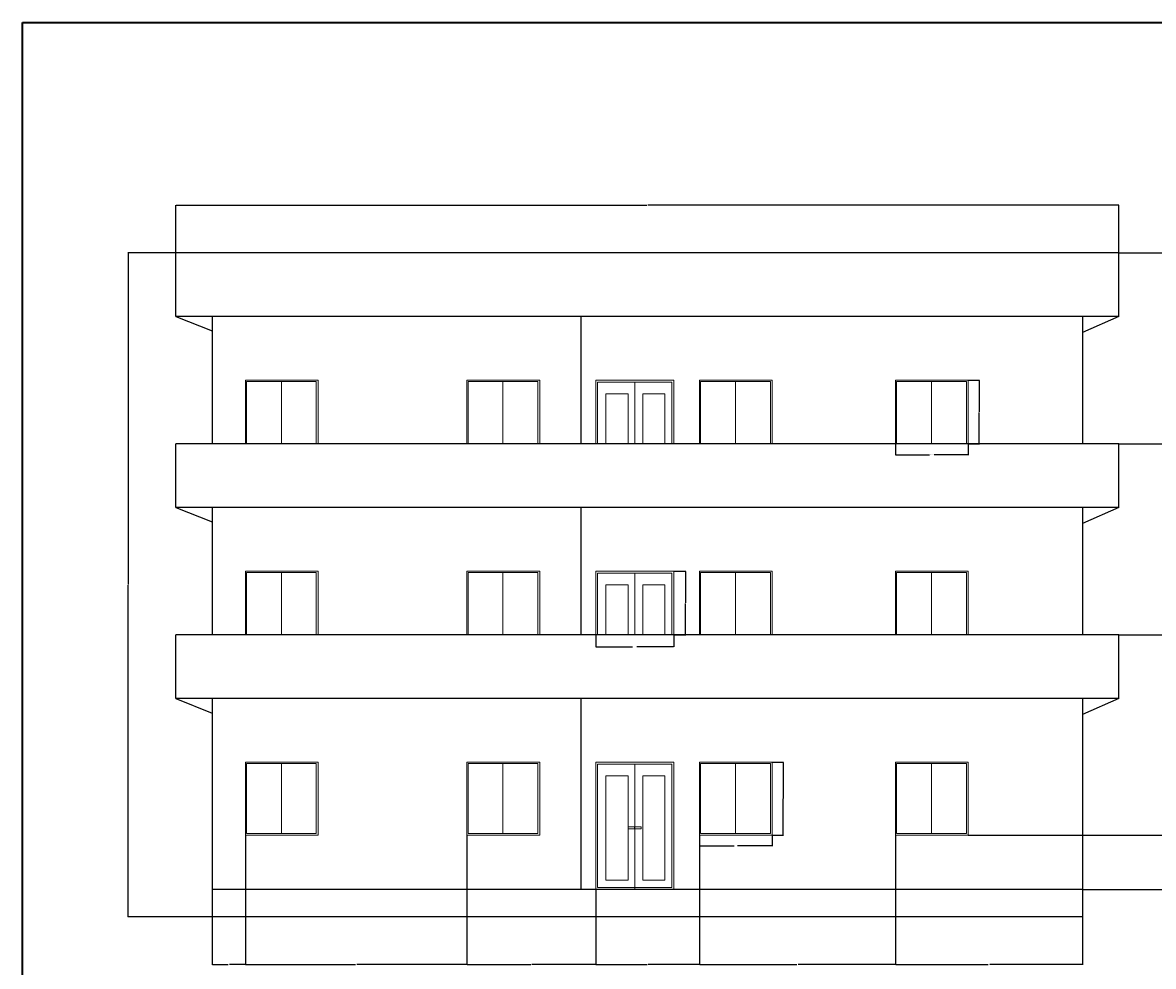
# Model space of a CAD drawing. Units: inches. Extents: x 1824 to 3509, y 619 to 2294.
# Tile 8 of 12: x 1824 to 2570, y 1671 to 2294. Entities that reach past the tile are written whole.
import ezdxf

# ---------------------------------------------------------------- set-up
doc = ezdxf.new("R2010")
doc.units = ezdxf.units.IN
for name, color, linetype, lineweight in [('A-ANNO-DIMS', 2, 'Continuous', 18), ('A-ANNO-TTLB', 7, 'Continuous', 35), ('A-ELEV', 7, 'Continuous', 25), ('A-ELEV-DOOR', 3, 'Continuous', 18), ('A-ELEV-GLAZ', 4, 'Continuous', 18)]:
    doc.layers.add(name, color=color, linetype=linetype, lineweight=lineweight)
doc.styles.get("Standard").update_dxf_attribs({"font": 'arial.ttf'})
doc.dimstyles.get("Standard").update_dxf_attribs({"dimtxt": 0.18, "dimasz": 0.18, "dimexe": 0.18, "dimexo": 0.0625, "dimgap": 0.09, "dimtad": 0, "dimtih": 1, "dimtoh": 1, "dimdec": 4, "dimzin": 0, "dimdsep": 46, "dimtxsty": 'Standard', "dimcen": 0.09, "dimadec": 0, "dimazin": 0, "dimtfac": 1, "dimtdec": 4, "dimtofl": 0, "dimtmove": 0, "dimatfit": 3, "dimfxl": 1, "dimtolj": 1, "dimtzin": 0, "dimarcsym": 0})

# ---------------------------------------------------------------- blocks, each defined once
blk = doc.blocks.new('WIN-ELEV-UPPER')
for p, q in [((0, 42), (0, 0)), ((48, 42), (0, 42)), ((23.74, 41.26), (23.74, 0)), ((48, 42), (48, 0))]:
    blk.add_line(p, q)
blk.add_lwpolyline([(0.72, 0), (0.72, 41.26), (46.77, 41.26), (46.77, 0)])
blk = doc.blocks.new('WIN-ELEV-48')
for p, q in [((0, 48), (0, 0)), ((48, 48), (0, 48)), ((23.74, 47.26), (23.74, 1.1)), ((48, 48), (48, 0)), ((48, 0), (0, 0))]:
    blk.add_line(p, q)
blk.add_lwpolyline([(0.72, 47.26), (46.77, 47.26), (46.77, 1.1), (0.72, 1.1)], close=True)
blk = doc.blocks.new('DOOR-ELEV-UPPER')
for p, q in [((0, 42), (0, 0)), ((51.54, 42), (0, 42)), ((25.72, 40.74), (25.72, 0)), ((51.54, 42), (51.54, 0))]:
    blk.add_line(p, q)
for points in [[(1.26, 0), (1.26, 40.74), (50.17, 40.74), (50.17, 0)], [(6.64, 0), (6.64, 33.08), (21.32, 33.08), (21.32, 0)], [(31.02, 0), (31.02, 33.08), (45.71, 33.08), (45.71, 0)]]:
    blk.add_lwpolyline(points)
blk = doc.blocks.new('*D36')
at = {"layer": 'A-ANNO-DIMS', "color": 0, "lineweight": -2, "transparency": 16777216}
for p, q in [((2399.66, 2015.69), (2399.66, 2008.37)), ((2447.66, 2015.69), (2447.66, 2008.37)), ((2399.84, 2008.55), (2422.08, 2008.55)), ((2447.48, 2008.55), (2425.24, 2008.55))]:
    blk.add_line(p, q, dxfattribs=at)
at = {"layer": 'A-ANNO-DIMS', "color": 0, "transparency": 16777216}
for points in [[(2399.84, 2008.58), (2399.84, 2008.52), (2399.66, 2008.55)], [(2447.48, 2008.58), (2447.48, 2008.52), (2447.66, 2008.55)]]:
    blk.add_solid(points, dxfattribs=at)
at = {"layer": 'Defpoints', "color": 0, "transparency": 16777216}
for p in [(2399.66, 2015.75), (2447.66, 2015.75), (2447.66, 2008.55)]:
    blk.add_point(p, dxfattribs=at)
at = {"layer": 'A-ANNO-DIMS', "color": 0, "transparency": 16777216, "insert": (2423.66, 2008.55), "char_height": 0.18, "attachment_point": 5}
blk.add_mtext('\\A1;UPPER WINDOW 48 TYP.', dxfattribs=at)
blk = doc.blocks.new('*D37')
at = {"layer": 'A-ANNO-DIMS', "color": 0, "lineweight": -2, "transparency": 16777216}
for p, q in [((2447.72, 2057.75), (2455.04, 2057.75)), ((2454.86, 2057.57), (2454.86, 2036.93)), ((2454.86, 2015.93), (2454.86, 2036.57)), ((2447.72, 2015.75), (2455.04, 2015.75))]:
    blk.add_line(p, q, dxfattribs=at)
at = {"layer": 'A-ANNO-DIMS', "color": 0, "transparency": 16777216}
for points in [[(2454.83, 2057.57), (2454.89, 2057.57), (2454.86, 2057.75)], [(2454.83, 2015.93), (2454.89, 2015.93), (2454.86, 2015.75)]]:
    blk.add_solid(points, dxfattribs=at)
at = {"layer": 'Defpoints', "color": 0, "transparency": 16777216}
for p in [(2447.66, 2057.75), (2454.86, 2057.75), (2447.66, 2015.75)]:
    blk.add_point(p, dxfattribs=at)
at = {"layer": 'A-ANNO-DIMS', "color": 0, "transparency": 16777216, "insert": (2454.86, 2036.75), "char_height": 0.18, "attachment_point": 5}
blk.add_mtext('\\A1;42 TYP.', dxfattribs=at)
blk = doc.blocks.new('*D46')
at = {"layer": 'A-ANNO-DIMS', "color": 0, "lineweight": -2, "transparency": 16777216}
for p, q in [((2270.48, 1757.69), (2270.48, 1750.37)), ((2318.48, 1757.69), (2318.48, 1750.37)), ((2270.66, 1750.55), (2293.37, 1750.55)), ((2318.3, 1750.55), (2295.6, 1750.55))]:
    blk.add_line(p, q, dxfattribs=at)
at = {"layer": 'A-ANNO-DIMS', "color": 0, "transparency": 16777216}
for points in [[(2270.66, 1750.58), (2270.66, 1750.52), (2270.48, 1750.55)], [(2318.3, 1750.58), (2318.3, 1750.52), (2318.48, 1750.55)]]:
    blk.add_solid(points, dxfattribs=at)
at = {"layer": 'Defpoints', "color": 0, "transparency": 16777216}
for p in [(2270.48, 1757.75), (2318.48, 1757.75), (2318.48, 1750.55)]:
    blk.add_point(p, dxfattribs=at)
at = {"layer": 'A-ANNO-DIMS', "color": 0, "transparency": 16777216, "insert": (2294.48, 1750.55), "char_height": 0.18, "attachment_point": 5}
blk.add_mtext('\\A1;WINDOW 48 TYP.', dxfattribs=at)
blk = doc.blocks.new('*D47')
at = {"layer": 'A-ANNO-DIMS', "color": 0, "lineweight": -2, "transparency": 16777216}
for p, q in [((2318.55, 1805.75), (2325.86, 1805.75)), ((2325.68, 1805.57), (2325.68, 1781.93)), ((2325.68, 1757.93), (2325.68, 1781.57)), ((2318.55, 1757.75), (2325.86, 1757.75))]:
    blk.add_line(p, q, dxfattribs=at)
at = {"layer": 'A-ANNO-DIMS', "color": 0, "transparency": 16777216}
for points in [[(2325.65, 1805.57), (2325.71, 1805.57), (2325.68, 1805.75)], [(2325.65, 1757.93), (2325.71, 1757.93), (2325.68, 1757.75)]]:
    blk.add_solid(points, dxfattribs=at)
at = {"layer": 'Defpoints', "color": 0, "transparency": 16777216}
for p in [(2318.48, 1805.75), (2325.68, 1805.75), (2318.48, 1757.75)]:
    blk.add_point(p, dxfattribs=at)
at = {"layer": 'A-ANNO-DIMS', "color": 0, "transparency": 16777216, "insert": (2325.68, 1781.75), "char_height": 0.18, "attachment_point": 5}
blk.add_mtext('\\A1;48 TYP.', dxfattribs=at)
blk = doc.blocks.new('*D86')
at = {"layer": 'A-ANNO-DIMS', "color": 0, "lineweight": -2, "transparency": 16777216}
for p, q in [((2201.98, 1889.69), (2201.98, 1881.84)), ((2253.53, 1889.69), (2253.53, 1881.84)), ((2202.16, 1882.02), (2226.35, 1882.02)), ((2253.35, 1882.02), (2229.16, 1882.02))]:
    blk.add_line(p, q, dxfattribs=at)
at = {"layer": 'A-ANNO-DIMS', "color": 0, "transparency": 16777216}
for points in [[(2202.16, 1882.05), (2202.16, 1881.99), (2201.98, 1882.02)], [(2253.35, 1882.05), (2253.35, 1881.99), (2253.53, 1882.02)]]:
    blk.add_solid(points, dxfattribs=at)
at = {"layer": 'Defpoints', "color": 0, "transparency": 16777216}
for p in [(2201.98, 1889.75), (2253.53, 1889.75), (2253.53, 1882.02)]:
    blk.add_point(p, dxfattribs=at)
at = {"layer": 'A-ANNO-DIMS', "color": 0, "transparency": 16777216, "insert": (2227.76, 1882.02), "char_height": 0.18, "attachment_point": 5}
blk.add_mtext('\\A1;UPPER DOOR 52 TYP.', dxfattribs=at)
blk = doc.blocks.new('*D87')
at = {"layer": 'A-ANNO-DIMS', "color": 0, "lineweight": -2, "transparency": 16777216}
for p, q in [((2253.59, 1931.75), (2261.44, 1931.75)), ((2261.26, 1931.57), (2261.26, 1910.93)), ((2261.26, 1889.93), (2261.26, 1910.57)), ((2253.59, 1889.75), (2261.44, 1889.75))]:
    blk.add_line(p, q, dxfattribs=at)
at = {"layer": 'A-ANNO-DIMS', "color": 0, "transparency": 16777216}
for points in [[(2261.23, 1931.57), (2261.29, 1931.57), (2261.26, 1931.75)], [(2261.23, 1889.93), (2261.29, 1889.93), (2261.26, 1889.75)]]:
    blk.add_solid(points, dxfattribs=at)
at = {"layer": 'Defpoints', "color": 0, "transparency": 16777216}
for p in [(2253.53, 1931.75), (2261.26, 1931.75), (2253.53, 1889.75)]:
    blk.add_point(p, dxfattribs=at)
at = {"layer": 'A-ANNO-DIMS', "color": 0, "transparency": 16777216, "insert": (2261.26, 1910.75), "char_height": 0.18, "attachment_point": 5}
blk.add_mtext('\\A1;42 TYP.', dxfattribs=at)
blk = doc.blocks.new('*D118')
at = {"layer": 'A-ANNO-DIMS', "color": 0, "lineweight": -2, "transparency": 16777216}
for p, q in [((1925.09, 2141.81), (1925.09, 2173.33)), ((1925.27, 2173.15), (2235.8, 2173.15)), ((2546.91, 2173.15), (2236.38, 2173.15)), ((2547.09, 2141.81), (2547.09, 2173.33))]:
    blk.add_line(p, q, dxfattribs=at)
at = {"layer": 'A-ANNO-DIMS', "color": 0, "transparency": 16777216}
for points in [[(1925.27, 2173.18), (1925.27, 2173.12), (1925.09, 2173.15)], [(2546.91, 2173.18), (2546.91, 2173.12), (2547.09, 2173.15)]]:
    blk.add_solid(points, dxfattribs=at)
at = {"layer": 'Defpoints', "color": 0, "transparency": 16777216}
for p in [(2547.09, 2173.15), (1925.09, 2141.75), (2547.09, 2141.75)]:
    blk.add_point(p, dxfattribs=at)
at = {"layer": 'A-ANNO-DIMS', "color": 0, "transparency": 16777216, "insert": (2236.09, 2173.15), "char_height": 0.18, "attachment_point": 5}
blk.add_mtext('\\A1;622', dxfattribs=at)
blk = doc.blocks.new('*D119')
at = {"layer": 'A-ANNO-DIMS', "color": 0, "lineweight": -2, "transparency": 16777216}
for p, q in [((1925.03, 2141.75), (1893.51, 2141.75)), ((1893.69, 2141.57), (1893.69, 1922.93)), ((1893.69, 1703.93), (1893.69, 1922.57)), ((1949.03, 1703.75), (1893.51, 1703.75))]:
    blk.add_line(p, q, dxfattribs=at)
at = {"layer": 'A-ANNO-DIMS', "color": 0, "transparency": 16777216}
for points in [[(1893.66, 2141.57), (1893.72, 2141.57), (1893.69, 2141.75)], [(1893.66, 1703.93), (1893.72, 1703.93), (1893.69, 1703.75)]]:
    blk.add_solid(points, dxfattribs=at)
at = {"layer": 'Defpoints', "color": 0, "transparency": 16777216}
for p in [(1893.69, 2141.75), (1925.09, 2141.75), (1949.09, 1703.75)]:
    blk.add_point(p, dxfattribs=at)
at = {"layer": 'A-ANNO-DIMS', "color": 0, "transparency": 16777216, "insert": (1893.69, 1922.75), "char_height": 0.18, "attachment_point": 5}
blk.add_mtext('\\A1;438', dxfattribs=at)
blk = doc.blocks.new('*D120')
at = {"layer": 'A-ANNO-DIMS', "color": 0, "lineweight": -2, "transparency": 16777216}
for p, q in [((1970.95, 1757.69), (1970.95, 1672.17)), ((1949.09, 1703.69), (1949.09, 1672.17)), ((1949.27, 1672.35), (1959.56, 1672.35)), ((1970.77, 1672.35), (1960.49, 1672.35))]:
    blk.add_line(p, q, dxfattribs=at)
at = {"layer": 'A-ANNO-DIMS', "color": 0, "transparency": 16777216}
for points in [[(1949.27, 1672.38), (1949.27, 1672.32), (1949.09, 1672.35)], [(1970.77, 1672.38), (1970.77, 1672.32), (1970.95, 1672.35)]]:
    blk.add_solid(points, dxfattribs=at)
at = {"layer": 'Defpoints', "color": 0, "transparency": 16777216}
for p in [(1970.95, 1757.75), (1949.09, 1703.75), (1970.95, 1672.35)]:
    blk.add_point(p, dxfattribs=at)
at = {"layer": 'A-ANNO-DIMS', "color": 0, "transparency": 16777216, "insert": (1960.02, 1672.35), "char_height": 0.18, "attachment_point": 5}
blk.add_mtext('\\A1;21.863', dxfattribs=at)
blk = doc.blocks.new('*D121')
at = {"layer": 'A-ANNO-DIMS', "color": 0, "lineweight": -2, "transparency": 16777216}
for p, q in [((1970.95, 1757.69), (1970.95, 1672.17)), ((2117.11, 1757.69), (2117.11, 1672.17)), ((1971.13, 1672.35), (2043.58, 1672.35)), ((2116.93, 1672.35), (2044.49, 1672.35))]:
    blk.add_line(p, q, dxfattribs=at)
at = {"layer": 'A-ANNO-DIMS', "color": 0, "transparency": 16777216}
for points in [[(1971.13, 1672.38), (1971.13, 1672.32), (1970.95, 1672.35)], [(2116.93, 1672.38), (2116.93, 1672.32), (2117.11, 1672.35)]]:
    blk.add_solid(points, dxfattribs=at)
at = {"layer": 'Defpoints', "color": 0, "transparency": 16777216}
for p in [(1970.95, 1757.75), (2117.11, 1757.75), (2117.11, 1672.35)]:
    blk.add_point(p, dxfattribs=at)
at = {"layer": 'A-ANNO-DIMS', "color": 0, "transparency": 16777216, "insert": (2044.03, 1672.35), "char_height": 0.18, "attachment_point": 5}
blk.add_mtext('\\A1;146.16', dxfattribs=at)
blk = doc.blocks.new('*D122')
at = {"layer": 'A-ANNO-DIMS', "color": 0, "lineweight": -2, "transparency": 16777216}
for p, q in [((2117.11, 1757.69), (2117.11, 1672.17)), ((2201.98, 1721.69), (2201.98, 1672.17)), ((2117.29, 1672.35), (2159.15, 1672.35)), ((2201.8, 1672.35), (2159.94, 1672.35))]:
    blk.add_line(p, q, dxfattribs=at)
at = {"layer": 'A-ANNO-DIMS', "color": 0, "transparency": 16777216}
for points in [[(2117.29, 1672.38), (2117.29, 1672.32), (2117.11, 1672.35)], [(2201.8, 1672.38), (2201.8, 1672.32), (2201.98, 1672.35)]]:
    blk.add_solid(points, dxfattribs=at)
at = {"layer": 'Defpoints', "color": 0, "transparency": 16777216}
for p in [(2117.11, 1757.75), (2201.98, 1721.75), (2201.98, 1672.35)]:
    blk.add_point(p, dxfattribs=at)
at = {"layer": 'A-ANNO-DIMS', "color": 0, "transparency": 16777216, "insert": (2159.55, 1672.35), "char_height": 0.18, "attachment_point": 5}
blk.add_mtext('\\A1;84.87', dxfattribs=at)
blk = doc.blocks.new('*D123')
at = {"layer": 'A-ANNO-DIMS', "color": 0, "lineweight": -2, "transparency": 16777216}
for p, q in [((2270.48, 1757.69), (2270.48, 1672.17)), ((2201.98, 1721.69), (2201.98, 1672.17)), ((2202.16, 1672.35), (2235.91, 1672.35)), ((2270.3, 1672.35), (2236.56, 1672.35))]:
    blk.add_line(p, q, dxfattribs=at)
at = {"layer": 'A-ANNO-DIMS', "color": 0, "transparency": 16777216}
for points in [[(2202.16, 1672.38), (2202.16, 1672.32), (2201.98, 1672.35)], [(2270.3, 1672.38), (2270.3, 1672.32), (2270.48, 1672.35)]]:
    blk.add_solid(points, dxfattribs=at)
at = {"layer": 'Defpoints', "color": 0, "transparency": 16777216}
for p in [(2270.48, 1757.75), (2201.98, 1721.75), (2270.48, 1672.35)]:
    blk.add_point(p, dxfattribs=at)
at = {"layer": 'A-ANNO-DIMS', "color": 0, "transparency": 16777216, "insert": (2236.23, 1672.35), "char_height": 0.18, "attachment_point": 5}
blk.add_mtext('\\A1;68.5', dxfattribs=at)
blk = doc.blocks.new('*D124')
at = {"layer": 'A-ANNO-DIMS', "color": 0, "lineweight": -2, "transparency": 16777216}
for p, q in [((2270.48, 1757.69), (2270.48, 1672.17)), ((2399.66, 1757.69), (2399.66, 1672.17)), ((2270.66, 1672.35), (2334.62, 1672.35)), ((2399.48, 1672.35), (2335.53, 1672.35))]:
    blk.add_line(p, q, dxfattribs=at)
at = {"layer": 'A-ANNO-DIMS', "color": 0, "transparency": 16777216}
for points in [[(2270.66, 1672.38), (2270.66, 1672.32), (2270.48, 1672.35)], [(2399.48, 1672.38), (2399.48, 1672.32), (2399.66, 1672.35)]]:
    blk.add_solid(points, dxfattribs=at)
at = {"layer": 'Defpoints', "color": 0, "transparency": 16777216}
for p in [(2270.48, 1757.75), (2399.66, 1757.75), (2399.66, 1672.35)]:
    blk.add_point(p, dxfattribs=at)
at = {"layer": 'A-ANNO-DIMS', "color": 0, "transparency": 16777216, "insert": (2335.07, 1672.35), "char_height": 0.18, "attachment_point": 5}
blk.add_mtext('\\A1;129.17', dxfattribs=at)
blk = doc.blocks.new('*D125')
at = {"layer": 'A-ANNO-DIMS', "color": 0, "lineweight": -2, "transparency": 16777216}
for p, q in [((2399.66, 1757.69), (2399.66, 1672.17)), ((2523.09, 1703.69), (2523.09, 1672.17)), ((2399.84, 1672.35), (2460.92, 1672.35)), ((2522.91, 1672.35), (2461.83, 1672.35))]:
    blk.add_line(p, q, dxfattribs=at)
at = {"layer": 'A-ANNO-DIMS', "color": 0, "transparency": 16777216}
for points in [[(2399.84, 1672.38), (2399.84, 1672.32), (2399.66, 1672.35)], [(2522.91, 1672.38), (2522.91, 1672.32), (2523.09, 1672.35)]]:
    blk.add_solid(points, dxfattribs=at)
at = {"layer": 'Defpoints', "color": 0, "transparency": 16777216}
for p in [(2399.66, 1757.75), (2523.09, 1703.75), (2523.09, 1672.35)]:
    blk.add_point(p, dxfattribs=at)
at = {"layer": 'A-ANNO-DIMS', "color": 0, "transparency": 16777216, "insert": (2461.37, 1672.35), "char_height": 0.18, "attachment_point": 5}
blk.add_mtext('\\A1;123.43', dxfattribs=at)
blk = doc.blocks.new('*D126')
at = {"layer": 'A-ANNO-DIMS', "color": 0, "lineweight": -2, "transparency": 16777216}
for p, q in [((2447.72, 1757.75), (2578.67, 1757.75)), ((2578.49, 1757.57), (2578.49, 1739.93)), ((2578.49, 1721.93), (2578.49, 1739.57)), ((2523.15, 1721.75), (2578.67, 1721.75))]:
    blk.add_line(p, q, dxfattribs=at)
at = {"layer": 'A-ANNO-DIMS', "color": 0, "transparency": 16777216}
for points in [[(2578.46, 1757.57), (2578.52, 1757.57), (2578.49, 1757.75)], [(2578.46, 1721.93), (2578.52, 1721.93), (2578.49, 1721.75)]]:
    blk.add_solid(points, dxfattribs=at)
at = {"layer": 'Defpoints', "color": 0, "transparency": 16777216}
for p in [(2447.66, 1757.75), (2578.49, 1757.75), (2523.09, 1721.75)]:
    blk.add_point(p, dxfattribs=at)
at = {"layer": 'A-ANNO-DIMS', "color": 0, "transparency": 16777216, "insert": (2578.49, 1739.75), "char_height": 0.18, "attachment_point": 5}
blk.add_mtext('\\A1;36', dxfattribs=at)
blk = doc.blocks.new('*D127')
at = {"layer": 'A-ANNO-DIMS', "color": 0, "lineweight": -2, "transparency": 16777216}
for p, q in [((2547.15, 1889.75), (2578.67, 1889.75)), ((2578.49, 1889.57), (2578.49, 1823.93)), ((2578.49, 1757.93), (2578.49, 1823.57)), ((2447.72, 1757.75), (2578.67, 1757.75))]:
    blk.add_line(p, q, dxfattribs=at)
at = {"layer": 'A-ANNO-DIMS', "color": 0, "transparency": 16777216}
for points in [[(2578.46, 1889.57), (2578.52, 1889.57), (2578.49, 1889.75)], [(2578.46, 1757.93), (2578.52, 1757.93), (2578.49, 1757.75)]]:
    blk.add_solid(points, dxfattribs=at)
at = {"layer": 'Defpoints', "color": 0, "transparency": 16777216}
for p in [(2547.09, 1889.75), (2578.49, 1889.75), (2447.66, 1757.75)]:
    blk.add_point(p, dxfattribs=at)
at = {"layer": 'A-ANNO-DIMS', "color": 0, "transparency": 16777216, "insert": (2578.49, 1823.75), "char_height": 0.18, "attachment_point": 5}
blk.add_mtext('\\A1;132', dxfattribs=at)
blk = doc.blocks.new('*D128')
at = {"layer": 'A-ANNO-DIMS', "color": 0, "lineweight": -2, "transparency": 16777216}
for p, q in [((2547.15, 2015.75), (2578.67, 2015.75)), ((2578.49, 2015.57), (2578.49, 1952.93)), ((2578.49, 1889.93), (2578.49, 1952.57)), ((2547.15, 1889.75), (2578.67, 1889.75))]:
    blk.add_line(p, q, dxfattribs=at)
at = {"layer": 'A-ANNO-DIMS', "color": 0, "transparency": 16777216}
for points in [[(2578.46, 2015.57), (2578.52, 2015.57), (2578.49, 2015.75)], [(2578.46, 1889.93), (2578.52, 1889.93), (2578.49, 1889.75)]]:
    blk.add_solid(points, dxfattribs=at)
at = {"layer": 'Defpoints', "color": 0, "transparency": 16777216}
for p in [(2547.09, 2015.75), (2578.49, 2015.75), (2547.09, 1889.75)]:
    blk.add_point(p, dxfattribs=at)
at = {"layer": 'A-ANNO-DIMS', "color": 0, "transparency": 16777216, "insert": (2578.49, 1952.75), "char_height": 0.18, "attachment_point": 5}
blk.add_mtext('\\A1;126', dxfattribs=at)
blk = doc.blocks.new('*D129')
at = {"layer": 'A-ANNO-DIMS', "color": 0, "lineweight": -2, "transparency": 16777216}
for p, q in [((2547.15, 2141.75), (2578.67, 2141.75)), ((2578.49, 2141.57), (2578.49, 2078.93)), ((2578.49, 2015.93), (2578.49, 2078.57)), ((2547.15, 2015.75), (2578.67, 2015.75))]:
    blk.add_line(p, q, dxfattribs=at)
at = {"layer": 'A-ANNO-DIMS', "color": 0, "transparency": 16777216}
for points in [[(2578.46, 2141.57), (2578.52, 2141.57), (2578.49, 2141.75)], [(2578.46, 2015.93), (2578.52, 2015.93), (2578.49, 2015.75)]]:
    blk.add_solid(points, dxfattribs=at)
at = {"layer": 'Defpoints', "color": 0, "transparency": 16777216}
for p in [(2547.09, 2141.75), (2578.49, 2141.75), (2547.09, 2015.75)]:
    blk.add_point(p, dxfattribs=at)
at = {"layer": 'A-ANNO-DIMS', "color": 0, "transparency": 16777216, "insert": (2578.49, 2078.75), "char_height": 0.18, "attachment_point": 5}
blk.add_mtext('\\A1;126', dxfattribs=at)

msp = doc.modelspace()

# ---------------------------------------------------------------- linework, layer by layer
at = {"layer": 'A-ANNO-TTLB'}
msp.add_lwpolyline([(1824.0608, 2293.6614), (3509.3484, 2293.6614), (3509.3484, 619.4665), (1824.0608, 619.4665)], close=True, dxfattribs=at)
at = {"layer": 'A-ELEV'}
for p, q in [((2547.0899, 2141.7521), (1925.0899, 2141.7521)), ((1925.0899, 2099.7521), (1925.0899, 2141.7521)), ((2547.0899, 2099.7521), (2547.0899, 2141.7521)), ((2547.0899, 2099.7521), (1925.0899, 2099.7521)), ((1925.0899, 2099.7521), (1949.0899, 2090.2691)), ((1949.0899, 2099.7521), (1949.0899, 2015.7521)), ((2192.0899, 2099.7521), (2192.0899, 2015.7521)), ((2523.0899, 2099.7521), (2523.0899, 2015.7521)), ((2547.0899, 2099.7521), (2523.0899, 2089.246)), ((2547.0899, 2099.7521), (2547.0899, 2099.7521)), ((2192.0899, 2093.7521), (2192.0899, 2015.7521)), ((2523.0899, 2089.246), (2523.0899, 2089.246)), ((2547.0899, 2015.7521), (1925.0899, 2015.7521)), ((2547.0899, 2015.7521), (1925.0899, 2015.7521)), ((1925.0899, 1973.7521), (1925.0899, 2015.7521)), ((2547.0899, 1973.7521), (2547.0899, 2015.7521)), ((2547.0899, 1973.7521), (1925.0899, 1973.7521)), ((2547.0899, 1973.7521), (1925.0899, 1973.7521)), ((1925.0899, 1973.7521), (1949.0899, 1964.2691)), ((1925.0899, 1973.7521), (1949.0899, 1964.2691)), ((1925.0899, 1973.7521), (1949.0899, 1964.2691)), ((1925.0899, 1973.7521), (1949.0899, 1964.2691)), ((1925.0899, 1973.7521), (1949.0899, 1964.2691)), ((1949.0899, 1973.7521), (1949.0899, 1889.7521)), ((1949.0899, 1973.7521), (1949.0899, 1889.7521)), ((1949.0899, 1973.7521), (1949.0899, 1955.7521)), ((2192.0899, 1973.7521), (2192.0899, 1889.7521)), ((2523.0899, 1973.7521), (2523.0899, 1889.7521)), ((2523.0899, 1973.7521), (2523.0899, 1889.7521)), ((2523.0899, 1973.7521), (2523.0899, 1955.7521)), ((2547.0899, 1973.7521), (2523.0899, 1963.246)), ((2547.0899, 1973.7521), (2523.0899, 1963.246)), ((2547.0899, 1973.7521), (2523.0899, 1963.246)), ((2547.0899, 1973.7521), (2523.0899, 1963.246)), ((2547.0899, 1973.7521), (2523.0899, 1963.246)), ((2192.0899, 1967.7521), (2192.0899, 1889.7521)), ((2192.0899, 1967.7521), (2192.0899, 1889.7521)), ((2192.0899, 1967.7521), (2192.0899, 1889.7521)), ((2547.0899, 1889.7521), (1925.0899, 1889.7521)), ((1925.0899, 1847.7521), (1925.0899, 1889.7521)), ((2547.0899, 1847.7521), (2547.0899, 1889.7521)), ((2547.0899, 1847.7521), (1925.0899, 1847.7521)), ((1925.0899, 1847.7521), (1949.0899, 1838.2691)), ((1949.0899, 1847.7521), (1949.0899, 1703.7521)), ((1949.0899, 1847.7521), (1949.0899, 1829.7521)), ((1949.0899, 1847.7521), (1949.0899, 1829.7521)), ((2192.0899, 1847.7521), (2192.0899, 1721.7521)), ((2523.0899, 1847.7521), (2523.0899, 1703.7521)), ((2523.0899, 1847.7521), (2523.0899, 1829.7521)), ((2523.0899, 1847.7521), (2523.0899, 1829.7521)), ((2547.0899, 1847.7521), (2523.0899, 1837.246)), ((2192.0899, 1841.7521), (2192.0899, 1721.7521)), ((2523.0899, 1721.7521), (1949.0899, 1721.7521)), ((2523.0899, 1703.7521), (1949.0899, 1703.7521)), ((2523.0899, 1703.7521), (1949.0899, 1703.7521))]:
    msp.add_line(p, q, dxfattribs=at)
at = {"layer": 'A-ELEV-DOOR'}
for p, q in [((2201.9846, 2057.7521), (2201.9846, 2015.7521)), ((2253.5256, 2057.7521), (2201.9846, 2057.7521)), ((2253.5256, 2057.7521), (2253.5256, 2015.7521)), ((2201.9846, 1931.7521), (2201.9846, 1889.7521)), ((2253.5256, 1931.7521), (2201.9846, 1931.7521)), ((2201.9846, 1931.7521), (2201.9846, 1889.7521)), ((2253.5256, 1931.7521), (2201.9846, 1931.7521)), ((2253.5256, 1931.7521), (2253.5256, 1889.7521)), ((2253.5256, 1931.7521), (2253.5256, 1889.7521)), ((2201.9846, 1805.7521), (2201.9846, 1721.7521)), ((2253.5256, 1805.7521), (2201.9846, 1805.7521)), ((2253.5256, 1805.7521), (2253.5256, 1721.7521)), ((2227.7004, 1804.4912), (2227.7004, 1721.7521))]:
    msp.add_line(p, q, dxfattribs=at)
for points in [[(2203.2429, 1804.4912), (2252.1579, 1804.4912), (2252.1579, 1723.0806), (2203.2429, 1723.0806)], [(2208.6237, 1796.8315), (2223.3062, 1796.8315), (2223.3062, 1727.9028), (2208.6237, 1727.9028)], [(2233.0077, 1796.8315), (2247.6903, 1796.8315), (2247.6903, 1727.9028), (2233.0077, 1727.9028)], [(2223.4506, 1763.1216), (2227.6889, 1763.1216), (2227.6889, 1761.765), (2223.4506, 1761.765)], [(2227.7004, 1763.1216), (2231.9387, 1763.1216), (2231.9387, 1761.765), (2227.7004, 1761.765)]]:
    msp.add_lwpolyline(points, close=True, dxfattribs=at)
at = {"layer": 'A-ELEV-GLAZ'}
for p, q in [((1970.9532, 2057.7521), (1970.9532, 2015.7521)), ((2018.9532, 2057.7521), (1970.9532, 2057.7521)), ((2018.9532, 2057.7521), (2018.9532, 2015.7521)), ((2117.1111, 2057.7521), (2117.1111, 2015.7521)), ((2165.1111, 2057.7521), (2117.1111, 2057.7521)), ((2117.1111, 2057.7521), (2117.1111, 2015.7521)), ((2165.1111, 2057.7521), (2117.1111, 2057.7521)), ((2165.1111, 2057.7521), (2165.1111, 2015.7521)), ((2165.1111, 2057.7521), (2165.1111, 2015.7521)), ((2165.1111, 2057.7521), (2165.1111, 2015.7521)), ((2165.1111, 2057.7521), (2165.1111, 2015.7521)), ((2270.4848, 2057.7521), (2270.4848, 2015.7521)), ((2318.4848, 2057.7521), (2270.4848, 2057.7521)), ((2270.4848, 2057.7521), (2270.4848, 2015.7521)), ((2318.4848, 2057.7521), (2270.4848, 2057.7521)), ((2318.4848, 2057.7521), (2318.4848, 2015.7521)), ((2318.4848, 2057.7521), (2318.4848, 2015.7521)), ((2399.6578, 2057.7521), (2399.6578, 2015.7521)), ((2447.6578, 2057.7521), (2399.6578, 2057.7521)), ((2399.6578, 2057.7521), (2399.6578, 2015.7521)), ((2447.6578, 2057.7521), (2399.6578, 2057.7521)), ((2447.6578, 2057.7521), (2447.6578, 2015.7521)), ((2447.6578, 2057.7521), (2447.6578, 2015.7521)), ((1970.9532, 1931.7521), (1970.9532, 1889.7521)), ((2018.9532, 1931.7521), (1970.9532, 1931.7521)), ((1970.9532, 1931.7521), (1970.9532, 1889.7521)), ((2018.9532, 1931.7521), (1970.9532, 1931.7521)), ((2018.9532, 1931.7521), (2018.9532, 1889.7521)), ((2018.9532, 1931.7521), (2018.9532, 1889.7521)), ((2117.1111, 1931.7521), (2117.1111, 1889.7521)), ((2165.1111, 1931.7521), (2117.1111, 1931.7521)), ((2117.1111, 1931.7521), (2117.1111, 1889.7521)), ((2165.1111, 1931.7521), (2117.1111, 1931.7521)), ((2117.1111, 1931.7521), (2117.1111, 1889.7521)), ((2165.1111, 1931.7521), (2117.1111, 1931.7521)), ((2165.1111, 1931.7521), (2165.1111, 1889.7521)), ((2165.1111, 1931.7521), (2165.1111, 1889.7521)), ((2165.1111, 1931.7521), (2165.1111, 1889.7521)), ((2165.1111, 1931.7521), (2165.1111, 1889.7521)), ((2165.1111, 1931.7521), (2165.1111, 1889.7521)), ((2165.1111, 1931.7521), (2165.1111, 1889.7521)), ((2270.4848, 1931.7521), (2270.4848, 1889.7521)), ((2318.4848, 1931.7521), (2270.4848, 1931.7521)), ((2270.4848, 1931.7521), (2270.4848, 1889.7521)), ((2318.4848, 1931.7521), (2270.4848, 1931.7521)), ((2270.4848, 1931.7521), (2270.4848, 1889.7521)), ((2318.4848, 1931.7521), (2270.4848, 1931.7521)), ((2318.4848, 1931.7521), (2318.4848, 1889.7521)), ((2318.4848, 1931.7521), (2318.4848, 1889.7521)), ((2318.4848, 1931.7521), (2318.4848, 1889.7521)), ((2399.6578, 1931.7521), (2399.6578, 1889.7521)), ((2447.6578, 1931.7521), (2399.6578, 1931.7521)), ((2399.6578, 1931.7521), (2399.6578, 1889.7521)), ((2447.6578, 1931.7521), (2399.6578, 1931.7521)), ((2399.6578, 1931.7521), (2399.6578, 1889.7521)), ((2447.6578, 1931.7521), (2399.6578, 1931.7521)), ((2447.6578, 1931.7521), (2447.6578, 1889.7521)), ((2447.6578, 1931.7521), (2447.6578, 1889.7521)), ((2447.6578, 1931.7521), (2447.6578, 1889.7521)), ((2117.1111, 1805.7521), (2117.1111, 1757.7521)), ((2165.1111, 1805.7521), (2117.1111, 1805.7521)), ((2165.1111, 1805.7521), (2165.1111, 1757.7521)), ((2165.1111, 1805.7521), (2165.1111, 1757.7521)), ((2270.4848, 1805.7521), (2270.4848, 1757.7521)), ((2318.4848, 1805.7521), (2270.4848, 1805.7521)), ((2318.4848, 1805.7521), (2318.4848, 1757.7521)), ((2399.6578, 1805.7521), (2399.6578, 1757.7521)), ((2447.6578, 1805.7521), (2399.6578, 1805.7521)), ((2447.6578, 1805.7521), (2447.6578, 1757.7521)), ((2165.1111, 1757.7521), (2117.1111, 1757.7521)), ((2318.4848, 1757.7521), (2270.4848, 1757.7521)), ((2447.6578, 1757.7521), (2399.6578, 1757.7521))]:
    msp.add_line(p, q, dxfattribs=at)

# ---------------------------------------------------------------- block references
at = {"layer": 'A-ELEV-DOOR'}
for p in [(2201.985, 2015.752), (2201.985, 1889.752)]:
    msp.add_blockref('DOOR-ELEV-UPPER', p, dxfattribs=at)
at = {"layer": 'A-ELEV-GLAZ'}
for name, p in [('WIN-ELEV-UPPER', (1970.953, 2015.752)), ('WIN-ELEV-UPPER', (2117.1109, 2015.752)), ('WIN-ELEV-UPPER', (2270.4846, 2015.752)), ('WIN-ELEV-UPPER', (2399.6576, 2015.752)), ('WIN-ELEV-UPPER', (1970.953, 1889.752)), ('WIN-ELEV-UPPER', (2117.1109, 1889.752)), ('WIN-ELEV-UPPER', (2270.4846, 1889.752)), ('WIN-ELEV-UPPER', (2399.6576, 1889.752)), ('WIN-ELEV-48', (1970.953, 1757.752)), ('WIN-ELEV-48', (2117.1109, 1757.752)), ('WIN-ELEV-48', (2270.4846, 1757.752)), ('WIN-ELEV-48', (2399.6576, 1757.752))]:
    msp.add_blockref(name, p, dxfattribs=at)

# ---------------------------------------------------------------- dimensions: what is measured, and where the dimension line sits
at = {"layer": 'A-ANNO-DIMS'}
for base, p1, p2, override, picture, middle in [((2547.0899, 2173.1521), (1925.0899, 2141.7521), (2547.0899, 2141.7521), {"dimdec": 0, "dimlfac": 1, "dimrnd": 0, "dimzin": 0, "dimdsep": 46, "dimlunit": 2}, '*D118', (2236.0899, 2173.1521)), ((1970.9532, 1672.3521), (1949.0899, 1703.7521), (1970.9532, 1757.7521), {"dimdec": 3, "dimlfac": 1, "dimrnd": 0, "dimzin": 0, "dimdsep": 46, "dimlunit": 2}, '*D120', (1960.0216, 1672.3521)), ((2117.1111, 1672.3521), (1970.9532, 1757.7521), (2117.1111, 1757.7521), {"dimdec": 2, "dimlfac": 1, "dimrnd": 0, "dimzin": 0, "dimdsep": 46, "dimlunit": 2}, '*D121', (2044.0321, 1672.3521)), ((2201.9846, 1672.3521), (2117.1111, 1757.7521), (2201.9846, 1721.7521), {"dimdec": 2, "dimlfac": 1, "dimrnd": 0, "dimzin": 0, "dimdsep": 46, "dimlunit": 2}, '*D122', (2159.5478, 1672.3521)), ((2270.4848, 1672.3521), (2201.9846, 1721.7521), (2270.4848, 1757.7521), {"dimdec": 1, "dimlfac": 1, "dimrnd": 0, "dimzin": 0, "dimdsep": 46, "dimlunit": 2}, '*D123', (2236.2347, 1672.3521)), ((2399.6578, 1672.3521), (2270.4848, 1757.7521), (2399.6578, 1757.7521), {"dimdec": 2, "dimlfac": 1, "dimrnd": 0, "dimzin": 0, "dimdsep": 46, "dimlunit": 2}, '*D124', (2335.0713, 1672.3521)), ((2523.0899, 1672.3521), (2399.6578, 1757.7521), (2523.0899, 1703.7521), {"dimdec": 2, "dimlfac": 1, "dimrnd": 0, "dimzin": 0, "dimdsep": 46, "dimlunit": 2}, '*D125', (2461.3739, 1672.3521))]:
    dim = msp.add_linear_dim(base=base, p1=p1, p2=p2, dimstyle='Standard', override=override, dxfattribs=at)
    dim.commit()
    dim.dimension.update_dxf_attribs({"geometry": picture, "text_midpoint": middle})
for base, p1, p2, picture, middle in [((1893.6899, 2141.7521), (1949.0899, 1703.7521), (1925.0899, 2141.7521), '*D119', (1893.6899, 1922.7521)), ((2578.4899, 2141.7521), (2547.0899, 2015.7521), (2547.0899, 2141.7521), '*D129', (2578.4899, 2078.7521)), ((2578.4899, 2015.7521), (2547.0899, 1889.7521), (2547.0899, 2015.7521), '*D128', (2578.4899, 1952.7521)), ((2578.4899, 1889.7521), (2447.6578, 1757.7521), (2547.0899, 1889.7521), '*D127', (2578.4899, 1823.7521)), ((2578.4899, 1757.7521), (2523.0899, 1721.7521), (2447.6578, 1757.7521), '*D126', (2578.4899, 1739.7521))]:
    dim = msp.add_linear_dim(base=base, p1=p1, p2=p2, angle=90, dimstyle='Standard', override={"dimdec": 0, "dimlfac": 1, "dimrnd": 0, "dimzin": 0, "dimdsep": 46, "dimlunit": 2}, dxfattribs=at)
    dim.commit()
    dim.dimension.update_dxf_attribs({"geometry": picture, "text_midpoint": middle})
for base, p1, p2, picture, middle in [((2454.8578, 2057.7521), (2447.6578, 2015.7521), (2447.6578, 2057.7521), '*D37', (2454.8578, 2036.7521)), ((2261.2568, 1931.7521), (2253.5256, 1889.7521), (2253.5256, 1931.7521), '*D87', (2261.2568, 1910.7521)), ((2325.6848, 1805.7521), (2318.4848, 1757.7521), (2318.4848, 1805.7521), '*D47', (2325.6848, 1781.7521))]:
    dim = msp.add_linear_dim(base=base, p1=p1, p2=p2, angle=90, text='<> TYP.', dimstyle='Standard', override={"dimdec": 0, "dimlfac": 1, "dimrnd": 0, "dimzin": 0, "dimdsep": 46, "dimlunit": 2}, dxfattribs=at)
    dim.commit()
    dim.dimension.update_dxf_attribs({"geometry": picture, "text_midpoint": middle})
for base, p1, p2, text, picture, middle in [((2447.6578, 2008.5521), (2399.6578, 2015.7521), (2447.6578, 2015.7521), 'UPPER WINDOW <> TYP.', '*D36', (2423.6578, 2008.5521)), ((2253.5256, 1882.0209), (2201.9846, 1889.7521), (2253.5256, 1889.7521), 'UPPER DOOR <> TYP.', '*D86', (2227.7551, 1882.0209)), ((2318.4848, 1750.5521), (2270.4848, 1757.7521), (2318.4848, 1757.7521), 'WINDOW <> TYP.', '*D46', (2294.4848, 1750.5521))]:
    dim = msp.add_linear_dim(base=base, p1=p1, p2=p2, text=text, dimstyle='Standard', override={"dimdec": 0, "dimlfac": 1, "dimrnd": 0, "dimzin": 0, "dimdsep": 46, "dimlunit": 2}, dxfattribs=at)
    dim.commit()
    dim.dimension.update_dxf_attribs({"geometry": picture, "text_midpoint": middle})

doc.saveas('drawing.dxf')
